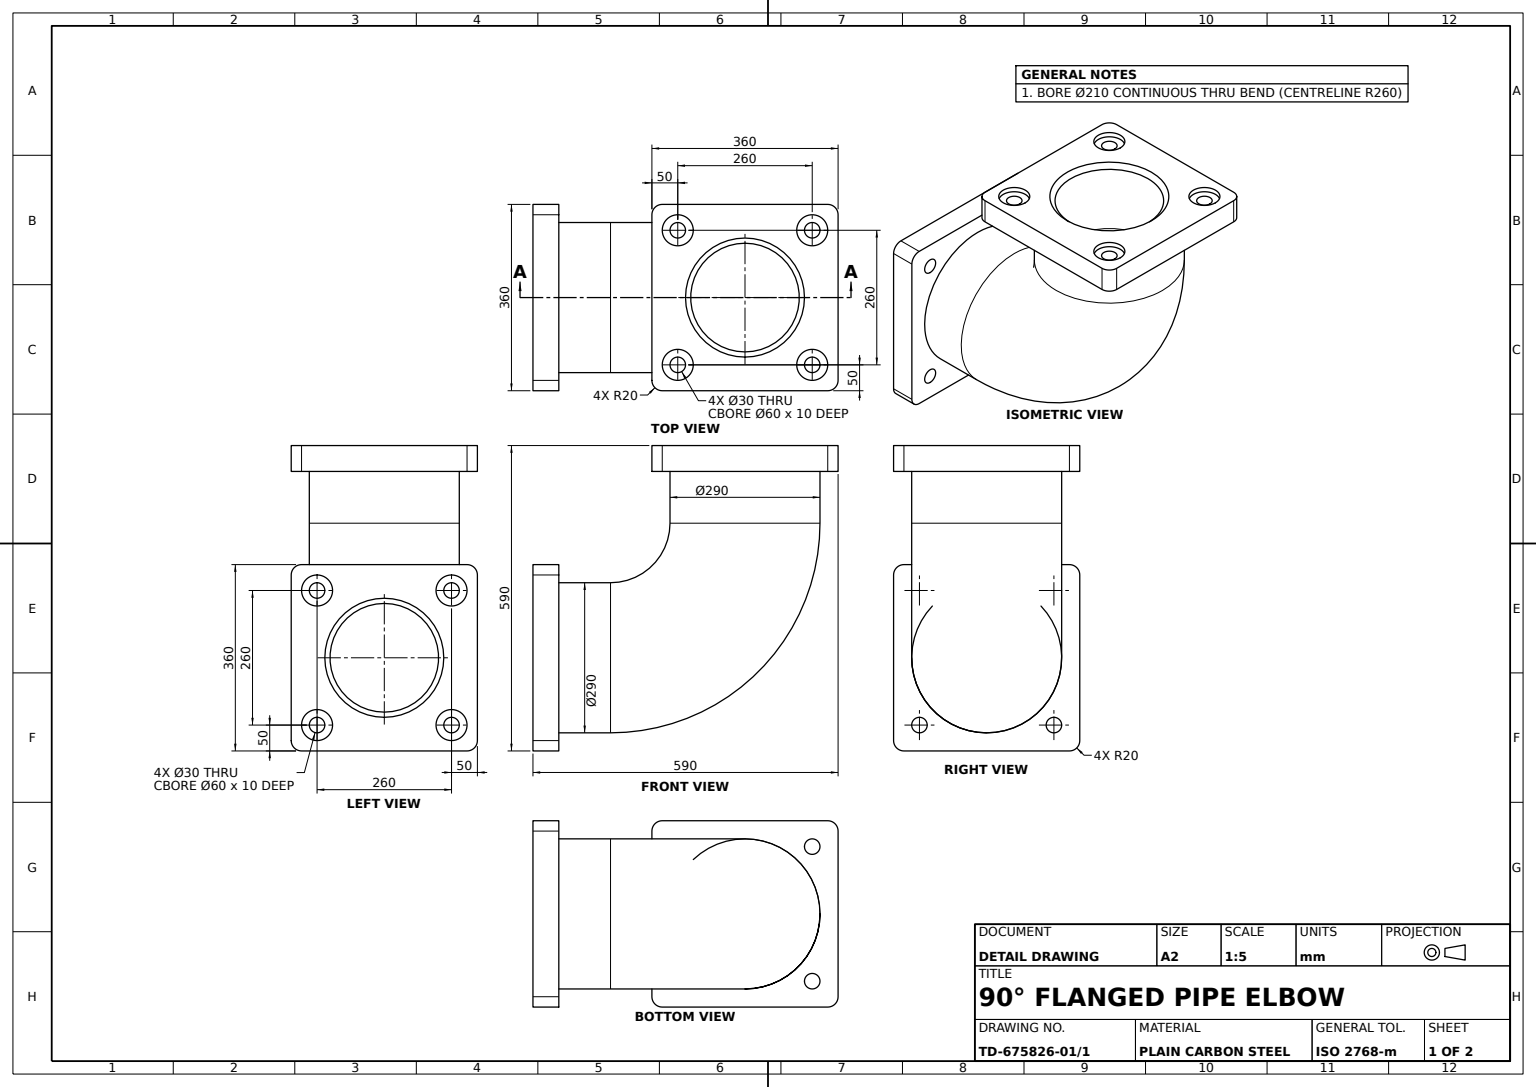
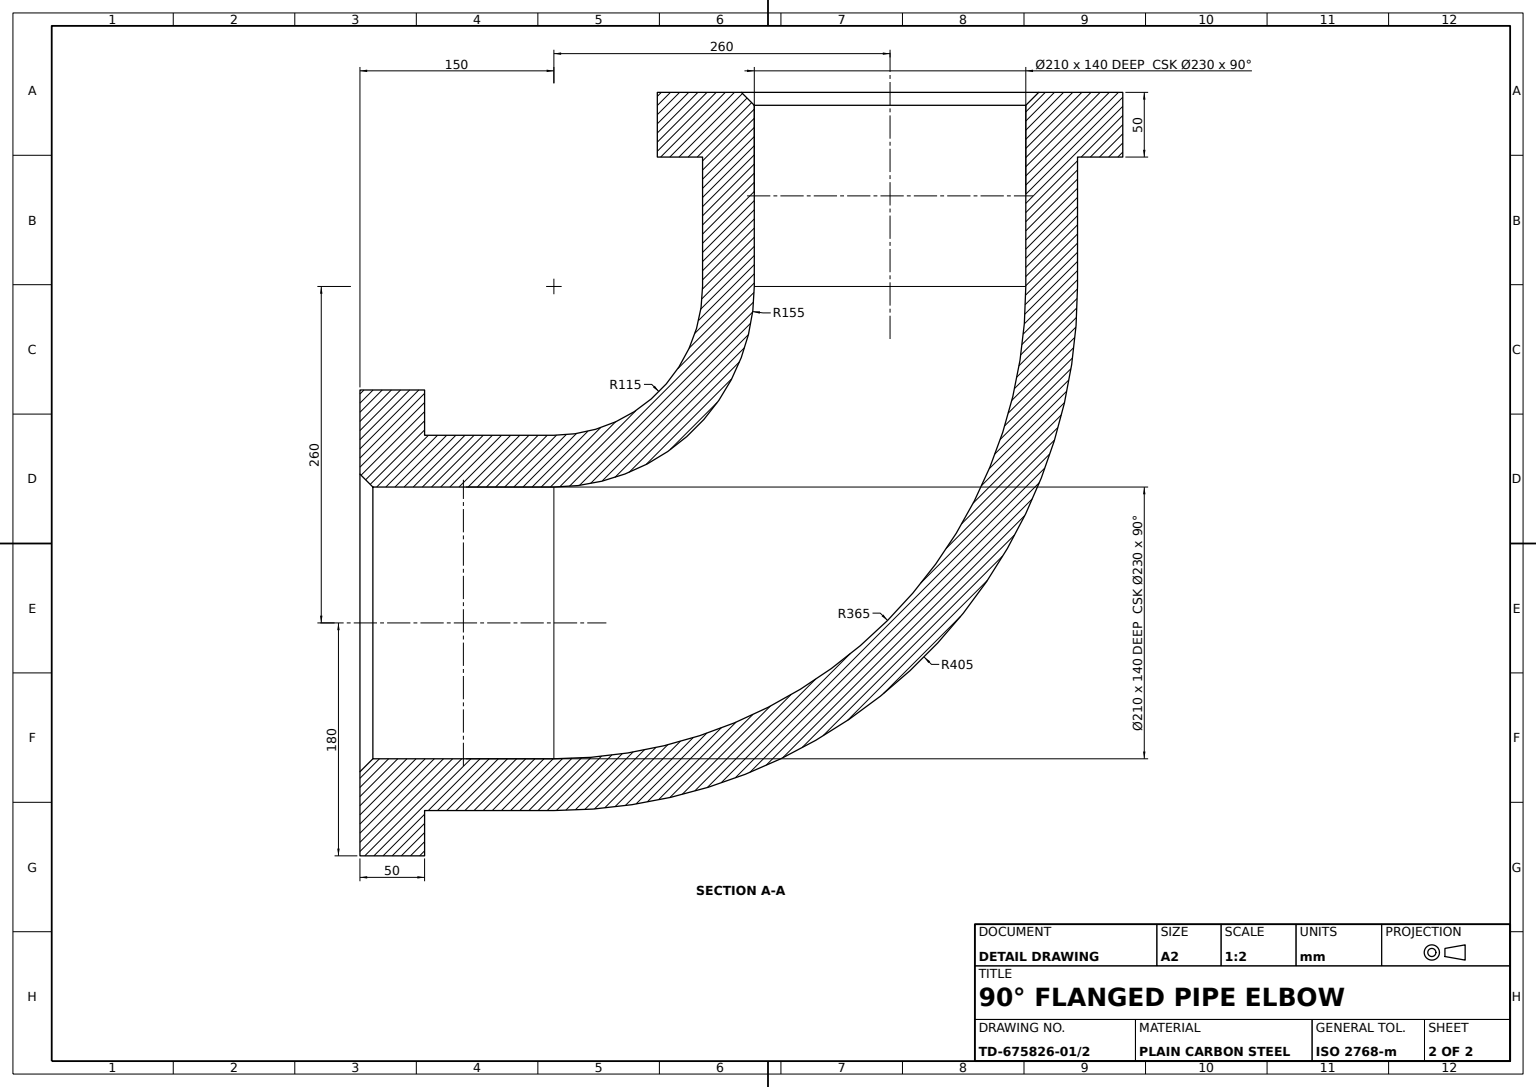
from build123d import *

# Parameters (mm, degrees)
ELBOW_PIPE_290_PROFILE_R          = 145
FLANGE_1_360X360X50_DEPTH         = 50
FLANGE_1_BOLT_HOLE_SKETCH_R       = 30
FLANGE_1_BOLT_HOLE_SKETCH_R_2     = 15
FLANGE_1_COUNTERBORES_4X_60_DEPTH = 10
SKETCH9_2_R                       = 15
FLANGE_1_BOLT_HOLES_4X_30_DEPTH   = 50
FLANGE_2_360X360X50_DEPTH         = 50
FLANGE_2_BOLT_HOLE_SKETCH_R       = 30
FLANGE_2_BOLT_HOLE_SKETCH_R_2     = 15
FLANGE_2_COUNTERBORES_4X_60_DEPTH = 10
SKETCH11_2_R                      = 15
FLANGE_2_BOLT_HOLES_4X_30_DEPTH   = 50
ELBOW_BORE_210_PROFILE_R          = 105
BORE_CHAMFER_10X45_SIZE           = 10


with BuildPart() as part:
    # Elbow Pipe _290: sweep along a path in Elbow Path Sketch
    with BuildLine(Plane.XY) as elbow_pipe_290_path:
        Line((0, 410), (0, 260))
        ThreePointArc((0, 260), (-76.152236891, 76.152236891), (-260, 0))
        Line((-260, 0), (-410, 0))
    # Elbow Pipe _290 profile (on start of the path) → Elbow Pipe _290 (sweep)
    with BuildSketch(Plane(origin=(0, 410, 0), x_dir=(0, 0, -1), z_dir=(0, -1, 0))):
        Circle(ELBOW_PIPE_290_PROFILE_R)
    sweep(path=elbow_pipe_290_path.line)

    # Flange 1 Sketch → Flange 1 360x360x50 (add)
    with BuildSketch(Plane(origin=(0, 410, 0), x_dir=(1, 0, 0), z_dir=(0, 1, 0))):
        with BuildLine():
            Line((-160, 180), (160, 180))
            ThreePointArc((160, 180), (174.142135624, 174.142135624), (180, 160))
            Line((180, 160), (180, -160))
            ThreePointArc((180, -160), (174.142135624, -174.142135624), (160, -180))
            Line((160, -180), (-160, -180))
            ThreePointArc((-160, -180), (-174.142135624, -174.142135624), (-180, -160))
            Line((-180, -160), (-180, 160))
            ThreePointArc((-180, 160), (-174.142135624, 174.142135624), (-160, 180))
        make_face()
    extrude(amount=-FLANGE_1_360X360X50_DEPTH)

    # Flange 1 Bolt Hole Sketch → Flange 1 Counterbores 4x_60 (cut)
    # profile 1 of 4: a face of its own
    with BuildSketch(Plane(origin=(0, 410, 0), x_dir=(1, 0, 0), z_dir=(0, 1, 0))):
        with Locations(Location((-130, 130, 0), (0, 0, 180))):
            Circle(FLANGE_1_BOLT_HOLE_SKETCH_R)
        with Locations(Location((-130, 130, 0), (0, 0, 180))):
            Circle(FLANGE_1_BOLT_HOLE_SKETCH_R_2, mode=Mode.SUBTRACT)
    # profile 2 of 4: a face of its own
    with BuildSketch(Plane(origin=(0, 410, 0), x_dir=(1, 0, 0), z_dir=(0, 1, 0))):
        with Locations(Location((-130, -130, 0), (0, 0, 180))):
            Circle(FLANGE_1_BOLT_HOLE_SKETCH_R)
        with Locations(Location((-130, -130, 0), (0, 0, 180))):
            Circle(FLANGE_1_BOLT_HOLE_SKETCH_R_2, mode=Mode.SUBTRACT)
    # profile 3 of 4: a face of its own
    with BuildSketch(Plane(origin=(0, 410, 0), x_dir=(1, 0, 0), z_dir=(0, 1, 0))):
        with Locations((130, -130)):
            Circle(FLANGE_1_BOLT_HOLE_SKETCH_R)
        with Locations((130, -130)):
            Circle(FLANGE_1_BOLT_HOLE_SKETCH_R_2, mode=Mode.SUBTRACT)
    # profile 4 of 4: a face of its own
    with BuildSketch(Plane(origin=(0, 410, 0), x_dir=(1, 0, 0), z_dir=(0, 1, 0))):
        with Locations((130, 130)):
            Circle(FLANGE_1_BOLT_HOLE_SKETCH_R)
        with Locations((130, 130)):
            Circle(FLANGE_1_BOLT_HOLE_SKETCH_R_2, mode=Mode.SUBTRACT)
    extrude(amount=-FLANGE_1_COUNTERBORES_4X_60_DEPTH, mode=Mode.SUBTRACT)

    # Sketch9_2 → Flange 1 Bolt Holes 4x_30 (cut)
    with BuildSketch(Plane(origin=(0, 410, 0), x_dir=(1, 0, 0), z_dir=(0, 1, 0))):
        with Locations(Location((-130, 130, 0), (0, 0, 180))):
            Circle(SKETCH9_2_R)
        with Locations(Location((130, 130, 0), (0, 0, 270))):
            Circle(SKETCH9_2_R)
        with Locations(Location((-130, -130, 0), (0, 0, 180))):
            Circle(SKETCH9_2_R)
        with Locations(Location((130, -130, 0), (0, 0, 270))):
            Circle(SKETCH9_2_R)
    extrude(amount=-FLANGE_1_BOLT_HOLES_4X_30_DEPTH, mode=Mode.SUBTRACT)

    # Flange 2 Sketch → Flange 2 360x360x50 (add)
    with BuildSketch(Plane.ZY.offset(410)):
        with BuildLine():
            Line((-160, 180), (160, 180))
            ThreePointArc((160, 180), (174.142135624, 174.142135624), (180, 160))
            Line((180, 160), (180, -160))
            ThreePointArc((180, -160), (174.142135624, -174.142135624), (160, -180))
            Line((160, -180), (-160, -180))
            ThreePointArc((-160, -180), (-174.142135624, -174.142135624), (-180, -160))
            Line((-180, -160), (-180, 160))
            ThreePointArc((-180, 160), (-174.142135624, 174.142135624), (-160, 180))
        make_face()
    extrude(amount=-FLANGE_2_360X360X50_DEPTH)

    # Flange 2 Bolt Hole Sketch → Flange 2 Counterbores 4x_60 (cut)
    # profile 1 of 4: a face of its own
    with BuildSketch(Plane.ZY.offset(410)):
        with Locations(Location((-130, 130, 0), (0, 0, 270))):
            Circle(FLANGE_2_BOLT_HOLE_SKETCH_R)
        with Locations(Location((-130, 130, 0), (0, 0, 270))):
            Circle(FLANGE_2_BOLT_HOLE_SKETCH_R_2, mode=Mode.SUBTRACT)
    # profile 2 of 4: a face of its own
    with BuildSketch(Plane.ZY.offset(410)):
        with Locations(Location((-130, -130, 0), (0, 0, 270))):
            Circle(FLANGE_2_BOLT_HOLE_SKETCH_R)
        with Locations(Location((-130, -130, 0), (0, 0, 270))):
            Circle(FLANGE_2_BOLT_HOLE_SKETCH_R_2, mode=Mode.SUBTRACT)
    # profile 3 of 4: a face of its own
    with BuildSketch(Plane.ZY.offset(410)):
        with Locations(Location((130, -130, 0), (0, 0, 90))):
            Circle(FLANGE_2_BOLT_HOLE_SKETCH_R)
        with Locations(Location((130, -130, 0), (0, 0, 90))):
            Circle(FLANGE_2_BOLT_HOLE_SKETCH_R_2, mode=Mode.SUBTRACT)
    # profile 4 of 4: a face of its own
    with BuildSketch(Plane.ZY.offset(410)):
        with Locations(Location((130, 130, 0), (0, 0, 90))):
            Circle(FLANGE_2_BOLT_HOLE_SKETCH_R)
        with Locations(Location((130, 130, 0), (0, 0, 90))):
            Circle(FLANGE_2_BOLT_HOLE_SKETCH_R_2, mode=Mode.SUBTRACT)
    extrude(amount=-FLANGE_2_COUNTERBORES_4X_60_DEPTH, mode=Mode.SUBTRACT)

    # Sketch11_2 → Flange 2 Bolt Holes 4x_30 (cut)
    with BuildSketch(Plane.ZY.offset(410)):
        with Locations(Location((130, 130, 0), (0, 0, 270))):
            Circle(SKETCH11_2_R)
        with Locations(Location((-130, 130, 0), (0, 0, 270))):
            Circle(SKETCH11_2_R)
        with Locations(Location((-130, -130, 0), (0, 0, 270))):
            Circle(SKETCH11_2_R)
        with Locations(Location((130, -130, 0), (0, 0, 90))):
            Circle(SKETCH11_2_R)
    extrude(amount=-FLANGE_2_BOLT_HOLES_4X_30_DEPTH, mode=Mode.SUBTRACT)

    # Elbow Bore _210: sweep along a path in Sketch1_2
    with BuildLine(Plane.XY) as elbow_bore_210_path:
        Line((0, 410), (0, 260))
        ThreePointArc((0, 260), (-76.152236891, 76.152236891), (-260, 0))
        Line((-260, 0), (-410, 0))
    # Elbow Bore _210 profile (on start of the path) → Elbow Bore _210 (sweep, cut)
    with BuildSketch(Plane(origin=(0, 410, 0), x_dir=(0, 0, -1), z_dir=(0, -1, 0))):
        Circle(ELBOW_BORE_210_PROFILE_R)
    sweep(path=elbow_bore_210_path.line, mode=Mode.SUBTRACT)

    # Bore Chamfer 10x45
    bore_chamfer_10x45_edges = [part.edges().sort_by_distance(p)[0] for p in [
        (-410, 0, 105),
        (0, 410, 105),
    ]]
    chamfer(bore_chamfer_10x45_edges, length=BORE_CHAMFER_10X45_SIZE)


solid = part.part
